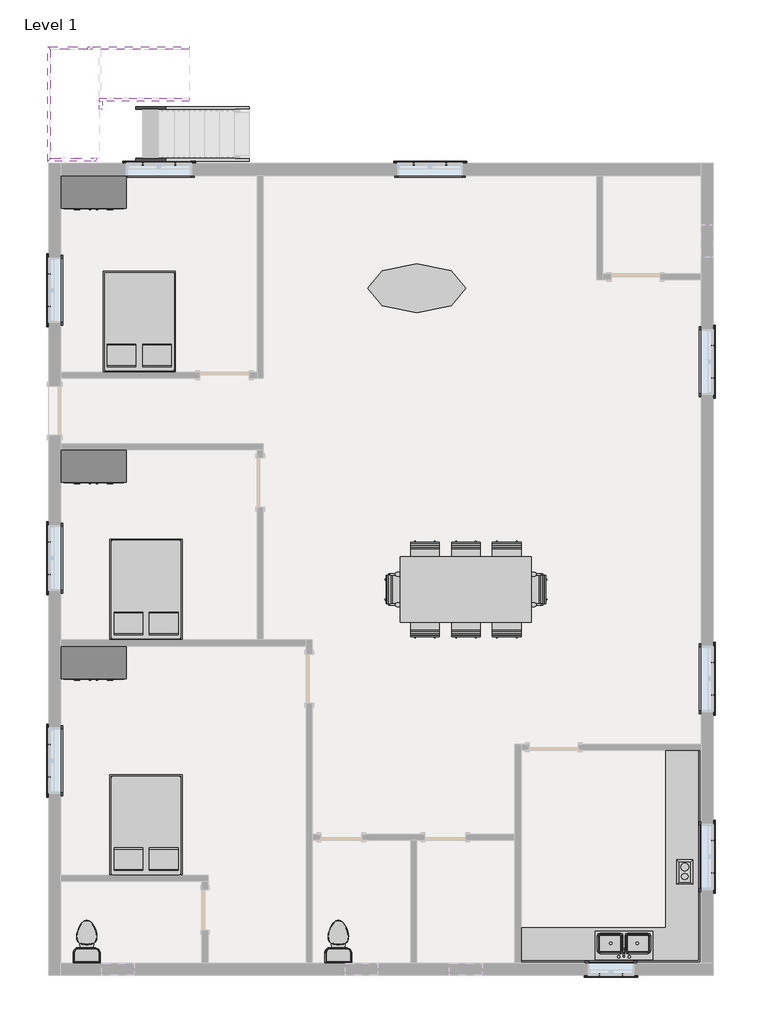
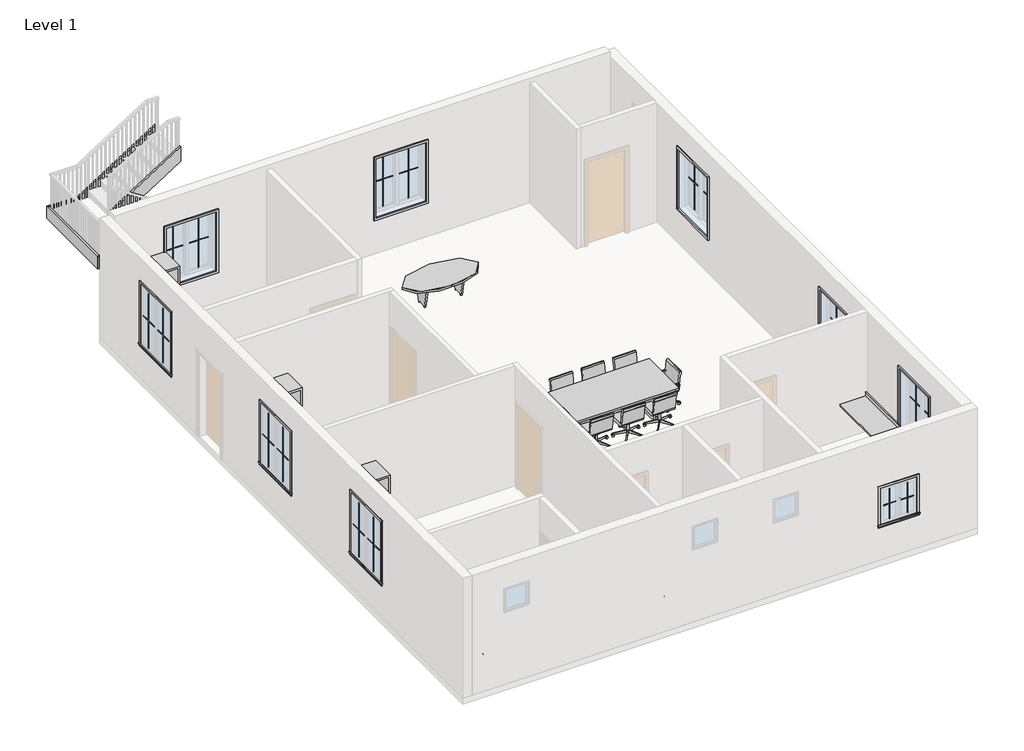
# One storey, part 3 of 3: 37 proxies, 17 furniture elements, 8 members, 3 flow terminals.
"""IFC4 building model written with IfcOpenShell, lengths in millimetres."""

from ifc_helpers import new_model, si_unit, frame, origin, place, context, project, spatial, polyline, outline, extrude, faceted_brep, transform, mapped, element, save
from components import proxy_fb8a77b2, muntin_pattern_2x2_muntin_pattern_2x2_6dad3731, muntin_pattern_2x2_muntin_pattern_2x2_a30a3345, muntin_pattern_2x2_muntin_pattern_2x2_b3fe6957, muntin_pattern_2x2_muntin_pattern_2x2_3e0ecaf2, trim_window_exterior_flat_with_sill_92b9b949, trim_window_exterior_flat_with_sill_41619996, trim_window_interior_flat_picture_frame_3bb882cf, trim_window_interior_flat_picture_frame_51c85655, flow_terminal_a53be723, toilet_domestic_3d_toilet_domestic_3d_ba6479b0, toilet_domestic_3d_toilet_domestic_3d_30431060, furniture_b58f7881, chair_task_chair_task_b7f3823b, chair_task_arms_chair_task_arms_fa5a08ef, furniture_9ea68cb4, furniture_6f689152, furniture_c045eb45, furniture_82e269c4

model = new_model("IFC4")

# Units and contexts
model_context = context("Model", 3, world=origin())
ifc_project = project(units=[si_unit("LENGTHUNIT", "METRE", prefix="MILLI")], contexts=[model_context])

# Site, building, storey
site = spatial("IfcSite", under=ifc_project)
building = spatial("IfcBuilding", under=site)
storey = spatial("IfcBuildingStorey", under=building, Name="Level 1", Elevation=0.0)

# Proxies
placement = place(None, origin())
proxy_shape = proxy_fb8a77b2(model_context)
element("IfcBuildingElementProxy", 1, Name="Cook Top-2 Unit : 12\" x 18\"", ObjectType="Cook Top-2 Unit : 12\" x 18\"", at=placement, inside=storey, context=model_context, shape_type="MappedRepresentation", body=[
    mapped(proxy_shape, transform((21379.2713581, 7569.2416109, 0.0), x_axis=(1.0, 0.0, 0.0), y_axis=(0.0, 1.0, 0.0), z_axis=(0.0, 0.0, 1.0))),
])
muntin_pattern_2x2_muntin_pattern_2x2_shape = muntin_pattern_2x2_muntin_pattern_2x2_6dad3731(model_context)
element("IfcBuildingElementProxy", 2, Name="Muntin Pattern_2x2 : Muntin Pattern_2x2", ObjectType="Muntin Pattern_2x2 : Muntin Pattern_2x2", at=placement, inside=storey, context=model_context, shape_type="MappedRepresentation", body=[
    mapped(muntin_pattern_2x2_muntin_pattern_2x2_shape, transform((9615.8963581, 18129.3539065, 984.25), x_axis=(0.0, 1.0, 0.0), y_axis=(-1.0, 0.0, 0.0), z_axis=(0.0, 0.0, 1.0))),
])
element("IfcBuildingElementProxy", 3, Name="Muntin Pattern_2x2 : Muntin Pattern_2x2", ObjectType="Muntin Pattern_2x2 : Muntin Pattern_2x2", at=placement, inside=storey, context=model_context, shape_type="MappedRepresentation", body=[
    mapped(muntin_pattern_2x2_muntin_pattern_2x2_shape, transform((11360.5588581, 20785.2414065, 984.25), x_axis=(1.0, 0.0, 0.0), y_axis=(0.0, 1.0, 0.0), z_axis=(0.0, 0.0, 1.0))),
])
element("IfcBuildingElementProxy", 4, Name="Muntin Pattern_2x2 : Muntin Pattern_2x2", ObjectType="Muntin Pattern_2x2 : Muntin Pattern_2x2", at=placement, inside=storey, context=model_context, shape_type="MappedRepresentation", body=[
    mapped(muntin_pattern_2x2_muntin_pattern_2x2_shape, transform((9615.8963581, 13138.2539065, 984.25), x_axis=(0.0, 1.0, 0.0), y_axis=(-1.0, 0.0, 0.0), z_axis=(0.0, 0.0, 1.0))),
])
element("IfcBuildingElementProxy", 5, Name="Muntin Pattern_2x2 : Muntin Pattern_2x2", ObjectType="Muntin Pattern_2x2 : Muntin Pattern_2x2", at=placement, inside=storey, context=model_context, shape_type="MappedRepresentation", body=[
    mapped(muntin_pattern_2x2_muntin_pattern_2x2_shape, transform((9615.8963581, 9366.3539065, 984.25), x_axis=(0.0, 1.0, 0.0), y_axis=(-1.0, 0.0, 0.0), z_axis=(0.0, 0.0, 1.0))),
])
element("IfcBuildingElementProxy", 6, Name="Muntin Pattern_2x2 : Muntin Pattern_2x2", ObjectType="Muntin Pattern_2x2 : Muntin Pattern_2x2", at=placement, inside=storey, context=model_context, shape_type="MappedRepresentation", body=[
    mapped(muntin_pattern_2x2_muntin_pattern_2x2_shape, transform((21979.3463581, 11496.7789065, 984.25), x_axis=(0.0, -1.0, 0.0), y_axis=(1.0, 0.0, 0.0), z_axis=(0.0, 0.0, 1.0))),
])
element("IfcBuildingElementProxy", 7, Name="Muntin Pattern_2x2 : Muntin Pattern_2x2", ObjectType="Muntin Pattern_2x2 : Muntin Pattern_2x2", at=placement, inside=storey, context=model_context, shape_type="MappedRepresentation", body=[
    mapped(muntin_pattern_2x2_muntin_pattern_2x2_shape, transform((21979.3463581, 17402.2789065, 984.25), x_axis=(0.0, -1.0, 0.0), y_axis=(1.0, 0.0, 0.0), z_axis=(0.0, 0.0, 1.0))),
])
element("IfcBuildingElementProxy", 8, Name="Muntin Pattern_2x2 : Muntin Pattern_2x2", ObjectType="Muntin Pattern_2x2 : Muntin Pattern_2x2", at=placement, inside=storey, context=model_context, shape_type="MappedRepresentation", body=[
    mapped(muntin_pattern_2x2_muntin_pattern_2x2_shape, transform((16408.8088581, 20785.2414065, 984.25), x_axis=(1.0, 0.0, 0.0), y_axis=(0.0, 1.0, 0.0), z_axis=(0.0, 0.0, 1.0))),
])
element("IfcBuildingElementProxy", 9, Name="Muntin Pattern_2x2 : Muntin Pattern_2x2", ObjectType="Muntin Pattern_2x2 : Muntin Pattern_2x2", at=placement, inside=storey, context=model_context, shape_type="MappedRepresentation", body=[
    mapped(muntin_pattern_2x2_muntin_pattern_2x2_shape, transform((21979.3463581, 8182.0789065, 984.25), x_axis=(0.0, -1.0, 0.0), y_axis=(1.0, 0.0, 0.0), z_axis=(0.0, 0.0, 1.0))),
])
muntin_pattern_2x2_muntin_pattern_2x2_2_shape = muntin_pattern_2x2_muntin_pattern_2x2_a30a3345(model_context)
element("IfcBuildingElementProxy", 10, Name="Muntin Pattern_2x2 : Muntin Pattern_2x2", ObjectType="Muntin Pattern_2x2 : Muntin Pattern_2x2", at=placement, inside=storey, context=model_context, shape_type="MappedRepresentation", body=[
    mapped(muntin_pattern_2x2_muntin_pattern_2x2_2_shape, transform((9615.8963581, 18735.7789065, 984.25), x_axis=(0.0, -1.0, 0.0), y_axis=(1.0, 0.0, 0.0), z_axis=(0.0, 0.0, 1.0))),
])
element("IfcBuildingElementProxy", 11, Name="Muntin Pattern_2x2 : Muntin Pattern_2x2", ObjectType="Muntin Pattern_2x2 : Muntin Pattern_2x2", at=placement, inside=storey, context=model_context, shape_type="MappedRepresentation", body=[
    mapped(muntin_pattern_2x2_muntin_pattern_2x2_2_shape, transform((11966.9838581, 20785.2414065, 984.25), x_axis=(-1.0, 0.0, 0.0), y_axis=(0.0, -1.0, 0.0), z_axis=(0.0, 0.0, 1.0))),
])
element("IfcBuildingElementProxy", 12, Name="Muntin Pattern_2x2 : Muntin Pattern_2x2", ObjectType="Muntin Pattern_2x2 : Muntin Pattern_2x2", at=placement, inside=storey, context=model_context, shape_type="MappedRepresentation", body=[
    mapped(muntin_pattern_2x2_muntin_pattern_2x2_2_shape, transform((9615.8963581, 13744.6789065, 984.25), x_axis=(0.0, -1.0, 0.0), y_axis=(1.0, 0.0, 0.0), z_axis=(0.0, 0.0, 1.0))),
])
element("IfcBuildingElementProxy", 13, Name="Muntin Pattern_2x2 : Muntin Pattern_2x2", ObjectType="Muntin Pattern_2x2 : Muntin Pattern_2x2", at=placement, inside=storey, context=model_context, shape_type="MappedRepresentation", body=[
    mapped(muntin_pattern_2x2_muntin_pattern_2x2_2_shape, transform((9615.8963581, 9972.7789065, 984.25), x_axis=(0.0, -1.0, 0.0), y_axis=(1.0, 0.0, 0.0), z_axis=(0.0, 0.0, 1.0))),
])
element("IfcBuildingElementProxy", 14, Name="Muntin Pattern_2x2 : Muntin Pattern_2x2", ObjectType="Muntin Pattern_2x2 : Muntin Pattern_2x2", at=placement, inside=storey, context=model_context, shape_type="MappedRepresentation", body=[
    mapped(muntin_pattern_2x2_muntin_pattern_2x2_2_shape, transform((21979.3463581, 10890.3539065, 984.25), x_axis=(0.0, 1.0, 0.0), y_axis=(-1.0, 0.0, 0.0), z_axis=(0.0, 0.0, 1.0))),
])
element("IfcBuildingElementProxy", 15, Name="Muntin Pattern_2x2 : Muntin Pattern_2x2", ObjectType="Muntin Pattern_2x2 : Muntin Pattern_2x2", at=placement, inside=storey, context=model_context, shape_type="MappedRepresentation", body=[
    mapped(muntin_pattern_2x2_muntin_pattern_2x2_2_shape, transform((21979.3463581, 16795.8539065, 984.25), x_axis=(0.0, 1.0, 0.0), y_axis=(-1.0, 0.0, 0.0), z_axis=(0.0, 0.0, 1.0))),
])
element("IfcBuildingElementProxy", 16, Name="Muntin Pattern_2x2 : Muntin Pattern_2x2", ObjectType="Muntin Pattern_2x2 : Muntin Pattern_2x2", at=placement, inside=storey, context=model_context, shape_type="MappedRepresentation", body=[
    mapped(muntin_pattern_2x2_muntin_pattern_2x2_2_shape, transform((17015.2338581, 20785.2414065, 984.25), x_axis=(-1.0, 0.0, 0.0), y_axis=(0.0, -1.0, 0.0), z_axis=(0.0, 0.0, 1.0))),
])
element("IfcBuildingElementProxy", 17, Name="Muntin Pattern_2x2 : Muntin Pattern_2x2", ObjectType="Muntin Pattern_2x2 : Muntin Pattern_2x2", at=placement, inside=storey, context=model_context, shape_type="MappedRepresentation", body=[
    mapped(muntin_pattern_2x2_muntin_pattern_2x2_2_shape, transform((21979.3463581, 7575.6539065, 984.25), x_axis=(0.0, 1.0, 0.0), y_axis=(-1.0, 0.0, 0.0), z_axis=(0.0, 0.0, 1.0))),
])
muntin_pattern_2x2_muntin_pattern_2x2_3_shape = muntin_pattern_2x2_muntin_pattern_2x2_b3fe6957(model_context)
element("IfcBuildingElementProxy", 18, Name="Muntin Pattern_2x2 : Muntin Pattern_2x2", ObjectType="Muntin Pattern_2x2 : Muntin Pattern_2x2", at=placement, inside=storey, context=model_context, shape_type="MappedRepresentation", body=[
    mapped(muntin_pattern_2x2_muntin_pattern_2x2_3_shape, transform((20298.1838581, 5678.5914065, 984.25), x_axis=(-1.0, 0.0, 0.0), y_axis=(0.0, -1.0, 0.0), z_axis=(0.0, 0.0, 1.0))),
])
muntin_pattern_2x2_muntin_pattern_2x2_4_shape = muntin_pattern_2x2_muntin_pattern_2x2_3e0ecaf2(model_context)
element("IfcBuildingElementProxy", 19, Name="Muntin Pattern_2x2 : Muntin Pattern_2x2", ObjectType="Muntin Pattern_2x2 : Muntin Pattern_2x2", at=placement, inside=storey, context=model_context, shape_type="MappedRepresentation", body=[
    mapped(muntin_pattern_2x2_muntin_pattern_2x2_4_shape, transform((19869.5588581, 5678.5914065, 984.25), x_axis=(1.0, 0.0, 0.0), y_axis=(0.0, 1.0, 0.0), z_axis=(0.0, 0.0, 1.0))),
])
trim_window_exterior_flat_with_sill_shape = trim_window_exterior_flat_with_sill_92b9b949(model_context)
element("IfcBuildingElementProxy", 20, Name="Trim-Window-Exterior-Flat : with Sill", ObjectType="Trim-Window-Exterior-Flat : with Sill", at=placement, inside=storey, context=model_context, shape_type="MappedRepresentation", body=[
    mapped(trim_window_exterior_flat_with_sill_shape, transform((9606.3713581, 18432.5664065, 2438.4), x_axis=(0.0, -1.0, 0.0), y_axis=(0.0, 0.0, 1.0), z_axis=(-1.0, 0.0, 0.0))),
])
element("IfcBuildingElementProxy", 21, Name="Trim-Window-Exterior-Flat : with Sill", ObjectType="Trim-Window-Exterior-Flat : with Sill", at=placement, inside=storey, context=model_context, shape_type="MappedRepresentation", body=[
    mapped(trim_window_exterior_flat_with_sill_shape, transform((11663.7713581, 20794.7664065, 2438.4), x_axis=(-1.0, 0.0, 0.0), y_axis=(0.0, 0.0, 1.0), z_axis=(0.0, 1.0, 0.0))),
])
element("IfcBuildingElementProxy", 22, Name="Trim-Window-Exterior-Flat : with Sill", ObjectType="Trim-Window-Exterior-Flat : with Sill", at=placement, inside=storey, context=model_context, shape_type="MappedRepresentation", body=[
    mapped(trim_window_exterior_flat_with_sill_shape, transform((9606.3713581, 13441.4664065, 2438.4), x_axis=(0.0, -1.0, 0.0), y_axis=(0.0, 0.0, 1.0), z_axis=(-1.0, 0.0, 0.0))),
])
element("IfcBuildingElementProxy", 23, Name="Trim-Window-Exterior-Flat : with Sill", ObjectType="Trim-Window-Exterior-Flat : with Sill", at=placement, inside=storey, context=model_context, shape_type="MappedRepresentation", body=[
    mapped(trim_window_exterior_flat_with_sill_shape, transform((9606.3713581, 9669.5664065, 2438.4), x_axis=(0.0, -1.0, 0.0), y_axis=(0.0, 0.0, 1.0), z_axis=(-1.0, 0.0, 0.0))),
])
element("IfcBuildingElementProxy", 24, Name="Trim-Window-Exterior-Flat : with Sill", ObjectType="Trim-Window-Exterior-Flat : with Sill", at=placement, inside=storey, context=model_context, shape_type="MappedRepresentation", body=[
    mapped(trim_window_exterior_flat_with_sill_shape, transform((21988.8713581, 11193.5664065, 2438.4), x_axis=(0.0, 1.0, 0.0), y_axis=(0.0, 0.0, 1.0), z_axis=(1.0, 0.0, 0.0))),
])
element("IfcBuildingElementProxy", 25, Name="Trim-Window-Exterior-Flat : with Sill", ObjectType="Trim-Window-Exterior-Flat : with Sill", at=placement, inside=storey, context=model_context, shape_type="MappedRepresentation", body=[
    mapped(trim_window_exterior_flat_with_sill_shape, transform((21988.8713581, 17099.0664065, 2438.4), x_axis=(0.0, 1.0, 0.0), y_axis=(0.0, 0.0, 1.0), z_axis=(1.0, 0.0, 0.0))),
])
element("IfcBuildingElementProxy", 26, Name="Trim-Window-Exterior-Flat : with Sill", ObjectType="Trim-Window-Exterior-Flat : with Sill", at=placement, inside=storey, context=model_context, shape_type="MappedRepresentation", body=[
    mapped(trim_window_exterior_flat_with_sill_shape, transform((16712.0213581, 20794.7664065, 2438.4), x_axis=(-1.0, 0.0, 0.0), y_axis=(0.0, 0.0, 1.0), z_axis=(0.0, 1.0, 0.0))),
])
element("IfcBuildingElementProxy", 27, Name="Trim-Window-Exterior-Flat : with Sill", ObjectType="Trim-Window-Exterior-Flat : with Sill", at=placement, inside=storey, context=model_context, shape_type="MappedRepresentation", body=[
    mapped(trim_window_exterior_flat_with_sill_shape, transform((21988.8713581, 7878.8664065, 2438.4), x_axis=(0.0, 1.0, 0.0), y_axis=(0.0, 0.0, 1.0), z_axis=(1.0, 0.0, 0.0))),
])
trim_window_exterior_flat_with_sill_2_shape = trim_window_exterior_flat_with_sill_41619996(model_context)
element("IfcBuildingElementProxy", 28, Name="Trim-Window-Exterior-Flat : with Sill", ObjectType="Trim-Window-Exterior-Flat : with Sill", at=placement, inside=storey, context=model_context, shape_type="MappedRepresentation", body=[
    mapped(trim_window_exterior_flat_with_sill_2_shape, transform((20083.8713581, 5669.0664065, 1828.8), x_axis=(1.0, 0.0, 0.0), y_axis=(0.0, 0.0, 1.0), z_axis=(0.0, -1.0, 0.0))),
])
trim_window_interior_flat_picture_frame_shape = trim_window_interior_flat_picture_frame_3bb882cf(model_context)
element("IfcBuildingElementProxy", 29, Name="Trim-Window-Interior-Flat : Picture Frame", ObjectType="Trim-Window-Interior-Flat : Picture Frame", at=placement, inside=storey, context=model_context, shape_type="MappedRepresentation", body=[
    mapped(trim_window_interior_flat_picture_frame_shape, transform((9834.9713581, 18432.5664065, 2438.4), x_axis=(0.0, 1.0, 0.0), y_axis=(0.0, 0.0, 1.0), z_axis=(1.0, 0.0, 0.0))),
])
element("IfcBuildingElementProxy", 30, Name="Trim-Window-Interior-Flat : Picture Frame", ObjectType="Trim-Window-Interior-Flat : Picture Frame", at=placement, inside=storey, context=model_context, shape_type="MappedRepresentation", body=[
    mapped(trim_window_interior_flat_picture_frame_shape, transform((11663.7713581, 20566.1664065, 2438.4), x_axis=(1.0, 0.0, 0.0), y_axis=(0.0, 0.0, 1.0), z_axis=(0.0, -1.0, 0.0))),
])
element("IfcBuildingElementProxy", 31, Name="Trim-Window-Interior-Flat : Picture Frame", ObjectType="Trim-Window-Interior-Flat : Picture Frame", at=placement, inside=storey, context=model_context, shape_type="MappedRepresentation", body=[
    mapped(trim_window_interior_flat_picture_frame_shape, transform((9834.9713581, 13441.4664065, 2438.4), x_axis=(0.0, 1.0, 0.0), y_axis=(0.0, 0.0, 1.0), z_axis=(1.0, 0.0, 0.0))),
])
element("IfcBuildingElementProxy", 32, Name="Trim-Window-Interior-Flat : Picture Frame", ObjectType="Trim-Window-Interior-Flat : Picture Frame", at=placement, inside=storey, context=model_context, shape_type="MappedRepresentation", body=[
    mapped(trim_window_interior_flat_picture_frame_shape, transform((9834.9713581, 9669.5664065, 2438.4), x_axis=(0.0, 1.0, 0.0), y_axis=(0.0, 0.0, 1.0), z_axis=(1.0, 0.0, 0.0))),
])
element("IfcBuildingElementProxy", 33, Name="Trim-Window-Interior-Flat : Picture Frame", ObjectType="Trim-Window-Interior-Flat : Picture Frame", at=placement, inside=storey, context=model_context, shape_type="MappedRepresentation", body=[
    mapped(trim_window_interior_flat_picture_frame_shape, transform((21760.2713581, 11193.5664065, 2438.4), x_axis=(0.0, -1.0, 0.0), y_axis=(0.0, 0.0, 1.0), z_axis=(-1.0, 0.0, 0.0))),
])
element("IfcBuildingElementProxy", 34, Name="Trim-Window-Interior-Flat : Picture Frame", ObjectType="Trim-Window-Interior-Flat : Picture Frame", at=placement, inside=storey, context=model_context, shape_type="MappedRepresentation", body=[
    mapped(trim_window_interior_flat_picture_frame_shape, transform((21760.2713581, 17099.0664065, 2438.4), x_axis=(0.0, -1.0, 0.0), y_axis=(0.0, 0.0, 1.0), z_axis=(-1.0, 0.0, 0.0))),
])
element("IfcBuildingElementProxy", 35, Name="Trim-Window-Interior-Flat : Picture Frame", ObjectType="Trim-Window-Interior-Flat : Picture Frame", at=placement, inside=storey, context=model_context, shape_type="MappedRepresentation", body=[
    mapped(trim_window_interior_flat_picture_frame_shape, transform((16712.0213581, 20566.1664065, 2438.4), x_axis=(1.0, 0.0, 0.0), y_axis=(0.0, 0.0, 1.0), z_axis=(0.0, -1.0, 0.0))),
])
element("IfcBuildingElementProxy", 36, Name="Trim-Window-Interior-Flat : Picture Frame", ObjectType="Trim-Window-Interior-Flat : Picture Frame", at=placement, inside=storey, context=model_context, shape_type="MappedRepresentation", body=[
    mapped(trim_window_interior_flat_picture_frame_shape, transform((21760.2713581, 7878.8664065, 2438.4), x_axis=(0.0, -1.0, 0.0), y_axis=(0.0, 0.0, 1.0), z_axis=(-1.0, 0.0, 0.0))),
])
trim_window_interior_flat_picture_frame_2_shape = trim_window_interior_flat_picture_frame_51c85655(model_context)
element("IfcBuildingElementProxy", 37, Name="Trim-Window-Interior-Flat : Picture Frame", ObjectType="Trim-Window-Interior-Flat : Picture Frame", at=placement, inside=storey, context=model_context, shape_type="MappedRepresentation", body=[
    mapped(trim_window_interior_flat_picture_frame_2_shape, transform((20083.8713581, 5897.6664065, 1828.8), x_axis=(-1.0, 0.0, 0.0), y_axis=(0.0, 0.0, 1.0), z_axis=(0.0, 1.0, 0.0))),
])

# Flow terminals
flow_terminal_shape = flow_terminal_a53be723(model_context)
element("IfcFlowTerminal", 38, ObjectType="Sink Kitchen-Double : 42\" x 21\"", at=placement, inside=storey, context=model_context, shape_type="MappedRepresentation", body=[
    mapped(flow_terminal_shape, transform((20340.8605987, 6230.2118076, 0.0), x_axis=(-1.0, 0.0, 0.0), y_axis=(0.0, -1.0, 0.0), z_axis=(0.0, 0.0, 1.0))),
])
toilet_domestic_3d_toilet_domestic_3d_shape = toilet_domestic_3d_toilet_domestic_3d_ba6479b0(model_context)
toilet_domestic_3d_toilet_domestic_3d_2_shape = toilet_domestic_3d_toilet_domestic_3d_30431060(model_context)
element("IfcFlowTerminal", 39, ObjectType="Toilet-Domestic-3D : Toilet-Domestic-3D", at=placement, inside=storey, context=model_context, shape_type="MappedRepresentation", body=[
    mapped(toilet_domestic_3d_toilet_domestic_3d_shape, transform((15003.8713581, 6392.3624338, 0.0), x_axis=(-1.0, 0.0, 0.0), y_axis=(0.0, -1.0, 0.0), z_axis=(0.0, 0.0, 1.0))),
    mapped(toilet_domestic_3d_toilet_domestic_3d_2_shape, transform((15003.8713581, 6392.3624338, 0.0), x_axis=(-1.0, 0.0, 0.0), y_axis=(0.0, -1.0, 0.0), z_axis=(0.0, 0.0, 1.0))),
])
element("IfcFlowTerminal", 40, ObjectType="Toilet-Domestic-3D : Toilet-Domestic-3D", at=placement, inside=storey, context=model_context, shape_type="MappedRepresentation", body=[
    mapped(toilet_domestic_3d_toilet_domestic_3d_shape, transform((10317.5713581, 6392.3624338, 0.0), x_axis=(-1.0, 0.0, 0.0), y_axis=(0.0, -1.0, 0.0), z_axis=(0.0, 0.0, 1.0))),
    mapped(toilet_domestic_3d_toilet_domestic_3d_2_shape, transform((10317.5713581, 6392.3624338, 0.0), x_axis=(-1.0, 0.0, 0.0), y_axis=(0.0, -1.0, 0.0), z_axis=(0.0, 0.0, 1.0))),
])

# Furniture
furniture_shape = furniture_b58f7881(model_context)
element("IfcFurniture", 41, ObjectType="Bed-Box : Double 53\" x 74\"", at=placement, inside=storey, context=model_context, shape_type="MappedRepresentation", body=[
    mapped(furniture_shape, transform((11636.4733436, 17613.9368983, 0.0), x_axis=(-1.0, 0.0, 0.0), y_axis=(0.0, -1.0, 0.0), z_axis=(0.0, 0.0, 1.0))),
])
element("IfcFurniture", 42, ObjectType="Bed-Box : Double 53\" x 74\"", at=placement, inside=storey, context=model_context, shape_type="MappedRepresentation", body=[
    mapped(furniture_shape, transform((11761.6238171, 12622.8368983, 0.0), x_axis=(-1.0, 0.0, 0.0), y_axis=(0.0, -1.0, 0.0), z_axis=(0.0, 0.0, 1.0))),
])
element("IfcFurniture", 43, ObjectType="Bed-Box : Double 53\" x 74\"", at=placement, inside=storey, context=model_context, shape_type="MappedRepresentation", body=[
    mapped(furniture_shape, transform((11761.6238171, 8228.6368983, 0.0), x_axis=(-1.0, 0.0, 0.0), y_axis=(0.0, -1.0, 0.0), z_axis=(0.0, 0.0, 1.0))),
])
chair_task_chair_task_shape = chair_task_chair_task_b7f3823b(model_context)
element("IfcFurniture", 44, ObjectType="Chair-Task : Chair-Task", at=placement, inside=storey, context=model_context, shape_type="MappedRepresentation", body=[
    mapped(chair_task_chair_task_shape, transform((17519.7621778, 13485.8123081, 0.0), x_axis=(-1.0, 0.0, 0.0), y_axis=(0.0, -1.0, 0.0), z_axis=(0.0, 0.0, 1.0))),
])
element("IfcFurniture", 45, ObjectType="Chair-Task : Chair-Task", at=placement, inside=storey, context=model_context, shape_type="MappedRepresentation", body=[
    mapped(chair_task_chair_task_shape, transform((18281.7621778, 13485.8123081, 0.0), x_axis=(-1.0, 0.0, 0.0), y_axis=(0.0, -1.0, 0.0), z_axis=(0.0, 0.0, 1.0))),
])
element("IfcFurniture", 46, ObjectType="Chair-Task : Chair-Task", at=placement, inside=storey, context=model_context, shape_type="MappedRepresentation", body=[
    mapped(chair_task_chair_task_shape, transform((17237.7805384, 12228.7205048, 0.0), x_axis=(1.0, 0.0, 0.0), y_axis=(0.0, 1.0, 0.0), z_axis=(0.0, 0.0, 1.0))),
])
element("IfcFurniture", 47, ObjectType="Chair-Task : Chair-Task", at=placement, inside=storey, context=model_context, shape_type="MappedRepresentation", body=[
    mapped(chair_task_chair_task_shape, transform((17999.7805384, 12228.7205048, 0.0), x_axis=(1.0, 0.0, 0.0), y_axis=(0.0, 1.0, 0.0), z_axis=(0.0, 0.0, 1.0))),
])
element("IfcFurniture", 48, ObjectType="Chair-Task : Chair-Task", at=placement, inside=storey, context=model_context, shape_type="MappedRepresentation", body=[
    mapped(chair_task_chair_task_shape, transform((16757.7621778, 13485.8123081, 0.0), x_axis=(-1.0, 0.0, 0.0), y_axis=(0.0, -1.0, 0.0), z_axis=(0.0, 0.0, 1.0))),
])
element("IfcFurniture", 49, ObjectType="Chair-Task : Chair-Task", at=placement, inside=storey, context=model_context, shape_type="MappedRepresentation", body=[
    mapped(chair_task_chair_task_shape, transform((16475.7805384, 12228.7205048, 0.0), x_axis=(1.0, 0.0, 0.0), y_axis=(0.0, 1.0, 0.0), z_axis=(0.0, 0.0, 1.0))),
])
chair_task_arms_chair_task_arms_shape = chair_task_arms_chair_task_arms_fa5a08ef(model_context)
element("IfcFurniture", 50, ObjectType="Chair-Task Arms : Chair-Task Arms", at=placement, inside=storey, context=model_context, shape_type="MappedRepresentation", body=[
    mapped(chair_task_arms_chair_task_arms_shape, transform((16140.6254565, 12998.2572261, 0.0), x_axis=(0.0, -1.0, 0.0), y_axis=(1.0, 0.0, 0.0), z_axis=(0.0, 0.0, 1.0))),
])
element("IfcFurniture", 51, ObjectType="Chair-Task Arms : Chair-Task Arms", at=placement, inside=storey, context=model_context, shape_type="MappedRepresentation", body=[
    mapped(chair_task_arms_chair_task_arms_shape, transform((18616.9172597, 12716.2755868, 0.0), x_axis=(0.0, 1.0, 0.0), y_axis=(-1.0, 0.0, 0.0), z_axis=(0.0, 0.0, 1.0))),
])
furniture_2_shape = furniture_9ea68cb4(model_context)
element("IfcFurniture", 52, ObjectType="Counter Top-L Shaped w Sink : 24\" Depth", at=placement, inside=storey, context=model_context, shape_type="MappedRepresentation", body=[
    mapped(furniture_2_shape, transform((20534.409063, 5923.0664065, 0.0), x_axis=(-1.0, 0.0, 0.0), y_axis=(0.0, -1.0, 0.0), z_axis=(0.0, 0.0, 1.0))),
])
furniture_3_shape = furniture_6f689152(model_context)
element("IfcFurniture", 53, ObjectType="Table-Conference2 w Chairs : 48\" x 144\"", at=placement, inside=storey, context=model_context, shape_type="MappedRepresentation", body=[
    mapped(furniture_3_shape, transform((17378.7713581, 12857.2664065, 0.0), x_axis=(1.0, 0.0, 0.0), y_axis=(0.0, 1.0, 0.0), z_axis=(0.0, 0.0, 1.0))),
])
furniture_4_shape = furniture_c045eb45(model_context)
element("IfcFurniture", 54, ObjectType="Table-Ellipse : 72\" x 36\"", at=placement, inside=storey, context=model_context, shape_type="MappedRepresentation", body=[
    mapped(furniture_4_shape, transform((16464.3713581, 18470.6664065, 0.0), x_axis=(1.0, 0.0, 0.0), y_axis=(0.0, 1.0, 0.0), z_axis=(0.0, 0.0, 1.0))),
])
furniture_5_shape = furniture_82e269c4(model_context)
element("IfcFurniture", 55, ObjectType="Wardrobe : 48\" x 72\" x 24\"", at=placement, inside=storey, context=model_context, shape_type="MappedRepresentation", body=[
    mapped(furniture_5_shape, transform((10713.7646179, 12082.105216, 0.0), x_axis=(1.0, 0.0, 0.0), y_axis=(0.0, 1.0, 0.0), z_axis=(0.0, 0.0, 1.0))),
])
element("IfcFurniture", 56, ObjectType="Wardrobe : 48\" x 72\" x 24\"", at=placement, inside=storey, context=model_context, shape_type="MappedRepresentation", body=[
    mapped(furniture_5_shape, transform((10713.7646179, 15739.705216, 0.0), x_axis=(1.0, 0.0, 0.0), y_axis=(0.0, 1.0, 0.0), z_axis=(0.0, 0.0, 1.0))),
])
element("IfcFurniture", 57, ObjectType="Wardrobe : 48\" x 72\" x 24\"", at=placement, inside=storey, context=model_context, shape_type="MappedRepresentation", body=[
    mapped(furniture_5_shape, transform((10713.7646179, 20845.105216, 0.0), x_axis=(1.0, 0.0, 0.0), y_axis=(0.0, 1.0, 0.0), z_axis=(0.0, 0.0, 1.0))),
])

# Members
element("IfcMember", 58, ObjectType="Stringer - 2\" Width", at=placement, inside=storey, context=model_context, shape_type="SweptSolid", body=[
    extrude(outline(polyline([(0.0, 13347.9752377), (215.0106437, 13347.9752377), (2032.0, 10492.7062492), (1727.2, 10403.9482797), (0.0, 13118.1197083), (0.0, 13347.9752377)])), frame((0.0, 20836.0384539, 0.0), z_axis=(0.0, 1.0, 0.0), x_axis=(0.0, 0.0, 1.0)), (0.0, 0.0, 1.0), 50.8),
])
element("IfcMember", 59, ObjectType="Stringer - 2\" Width", at=placement, inside=storey, context=model_context, shape_type="SweptSolid", body=[
    extrude(outline(polyline([(0.0, 13347.9752377), (215.0106437, 13347.9752377), (1960.683371, 10604.7752377), (1599.4010268, 10604.7752377), (0.0, 13118.1197083), (0.0, 13347.9752377)])), frame((0.0, 21801.2384539, 0.0), z_axis=(0.0, 1.0, 0.0), x_axis=(0.0, 0.0, 1.0)), (0.0, 0.0, 1.0), 50.8),
])
element("IfcMember", 60, ObjectType="Stringer - 2\" Width", at=placement, inside=storey, context=model_context, shape_type="SweptSolid", body=[
    extrude(outline(polyline([(2032.0, 10335.8442261), (1727.2, 10424.6021956), (2876.3282995, 12230.3752377), (3237.6106437, 12230.3752377), (2032.0, 10335.8442261)])), frame((0.0, 22920.6919009, 0.0), z_axis=(0.0, 1.0, 0.0), x_axis=(0.0, 0.0, 1.0)), (0.0, 0.0, 1.0), 50.8),
])
element("IfcMember", 61, ObjectType="Stringer - 2\" Width", at=placement, inside=storey, context=model_context, shape_type="SweptSolid", body=[
    extrude(outline(polyline([(2170.8106437, 10553.9752377), (1809.5282995, 10553.9752377), (2876.3282995, 12230.3752377), (3237.6106437, 12230.3752377), (2170.8106437, 10553.9752377)])), frame((0.0, 21955.4919009, 0.0), z_axis=(0.0, 1.0, 0.0), x_axis=(0.0, 0.0, 1.0)), (0.0, 0.0, 1.0), 50.8),
])
element("IfcMember", 62, ObjectType="Stringer - 2\" Width", at=placement, inside=storey, context=model_context, shape_type="Brep", body=[
    faceted_brep([(10335.8442261, 22920.6919009, 2032.0), (10335.8442261, 22971.4919009, 2032.0), (9588.7752377, 22971.4919009, 2032.0), (9639.5752377, 22920.6919009, 2032.0), (10424.6021956, 22920.6919009, 1727.2), (9639.5752377, 22920.6919009, 1727.2), (10424.6021956, 22971.4919009, 1727.2), (9588.7752377, 22971.4919009, 1727.2)], [[[0, 1, 2, 3]], [[4, 0, 3, 5]], [[6, 4, 5, 7]], [[1, 6, 7, 2]], [[1, 0, 4, 6]], [[2, 7, 5, 3]]]),
])
element("IfcMember", 63, ObjectType="Stringer - 2\" Width", at=placement, inside=storey, context=model_context, shape_type="SweptSolid", body=[
    extrude(outline(polyline([(9588.7752377, 22971.4919009), (9639.5752377, 22920.6919009), (9639.5752377, 20886.8384539), (9588.7752377, 20836.0384539), (9588.7752377, 22971.4919009)])), frame((0.0, 0.0, 1727.2), z_axis=(0.0, 0.0, 1.0), x_axis=(1.0, 0.0, 0.0)), (0.0, 0.0, 1.0), 304.8),
])
element("IfcMember", 64, ObjectType="Stringer - 2\" Width", at=placement, inside=storey, context=model_context, shape_type="Brep", body=[
    faceted_brep([(9639.5752377, 20886.8384539, 2032.0), (9588.7752377, 20836.0384539, 2032.0), (10492.7062492, 20836.0384539, 2032.0), (10492.7062492, 20886.8384539, 2032.0), (9639.5752377, 20886.8384539, 1727.2), (10403.9482797, 20886.8384539, 1727.2), (9588.7752377, 20836.0384539, 1727.2), (10403.9482797, 20836.0384539, 1727.2)], [[[0, 1, 2, 3]], [[4, 0, 3, 5]], [[6, 4, 5, 7]], [[1, 6, 7, 2]], [[1, 0, 4, 6]], [[2, 7, 5, 3]]]),
])
element("IfcMember", 65, ObjectType="Stringer - 2\" Width", at=placement, inside=storey, context=model_context, shape_type="SweptSolid", body=[
    extrude(outline(polyline([(10604.7752377, 21801.2384539), (10553.9752377, 21801.2384539), (10553.9752377, 21955.4919009), (10604.7752377, 21955.4919009), (10604.7752377, 21801.2384539)])), frame((0.0, 0.0, 1727.2), z_axis=(0.0, 0.0, 1.0), x_axis=(1.0, 0.0, 0.0)), (0.0, 0.0, 1.0), 304.8),
])

save(model, "model.ifc")

# Revit data of these elements
# Type "Cook Top-2 Unit : 12\" x 18\""
#   Assembly Code = "E1090400"
#   Counter Height = 3' - 0"
#   Depth = 1' - 6"
#   Width = 1' - 0"
#   Burner Material = Metal - Chrome
#   Cooktop Material = Metal - Steel, Polished
#   Default Elevation = 0
# Type "Muntin Pattern_2x2 : Muntin Pattern_2x2"
#   Width [instance default] = 4' - 0"
#   Thickness = 0' - 0 1/2"
#   Height [instance default] = 4' - 0"
#   Distance = 0' - 0 3/4"
#   Interior Material [instance default] = none
#   Exterior Material [instance default] = none
#   Default Elevation = 0
# Type "Trim-Window-Exterior-Flat : with Sill"
#   Trim Width = 0' - 2 1/4"
#   Trim Thickness_Picture Frame = 0' - 1 1/4"
#   Trim Thickness_with Sill = 0' - 0 3/4"
#   Sill Thickness = 0' - 1 1/4"
#   Opening Width [instance default] = 2' - 0"
#   Opening Height [instance default] = 3' - 0"
#   Default Elevation = 4' - 0"
#   Sill = yes
#   Picture Frame = no
#   Trim Material [instance default] = none
# Type "Trim-Window-Interior-Flat : Picture Frame"
#   Trim Thickness_Picture Frame = 0' - 1 1/4"
#   Trim Width = 0' - 2 1/4"
#   Trim Thickness_with Sill = 0' - 0 3/4"
#   Sill Thickness = 0' - 1 1/4"
#   Opening Width [instance default] = 2' - 0"
#   Opening Height [instance default] = 3' - 0"
#   Default Elevation = 4' - 0"
#   Sill = no
#   Picture Frame = yes
#   Trim Material [instance default] = none
# Type "Sink Kitchen-Double : 42\" x 21\""
#   Assembly Code = "D2010410"
#   Counter Height = 3' - 0"
#   Depth = 1' - 9"
#   Width = 3' - 6"
#   Faucet Material = Steel, Polished
#   Sink Material = Steel, Polished
#   Default Elevation = 0
# Type "Toilet-Domestic-3D : Toilet-Domestic-3D"
#   Assembly Code = "D2010110"
#   Toilet - Bowl/Basin Material = Porcelain, Linen
#   Toilet - Seat Material = Laminate, Linen, Matte
#   Default Elevation = 0
# Type "Bed-Box : Double 53\" x 74\""
#   Assembly Code = "E2020200"
#   Length = 6' - 2"
#   Width = 4' - 5"
#   Frame Material = Birch
#   Mattress Material = Linen, White
#   Default Elevation = 0
# Type "Chair-Task : Chair-Task"
#   Assembly Code = "E2020200"
#   Base Material = Plastic - Black
#   Caster Material = Plastic - Black
#   Seat/Back Material = Textile - Slate Blue
#   Default Elevation = 0
# Type "Chair-Task Arms : Chair-Task Arms"
#   Assembly Code = "E2020200"
#   Base Material = Plastic - Black
#   Caster Material = Plastic - Black
#   Seat/Back Material = Textile - Slate Blue
#   Default Elevation = 0
# Type "Counter Top-L Shaped w Sink : 24\" Depth"
#   Assembly Code = "C1030400"
#   Counter Thickness = 0' - 1 1/2"
#   Depth = 2' - 1"
#   Height = 3' - 0"
#   Length - Leg 1 [instance default] = 8' - 0"
#   Length - Leg 2 [instance default] = 6' - 0"
#   Sink Location [instance default] = 3' - 0"
#   Sink Location To Wall [instance default] = 0' - 6"
#   Sink Opening Depth [instance default] = 1' - 3"
#   Sink Opening Width [instance default] = 3' - 3"
#   Counter Top Material = none
#   Default Elevation = 0
# Type "Table-Conference2 w Chairs : 48\" x 144\""
#   Assembly Code = "E2020200"
#   Description = "Seating 12-14"
#   Height = 2' - 6"
#   Length = 8' - 0"
#   Width = 4' - 0"
#   Number Of Chairs One Side = 3
#   Number Of Chairs = 8
#   Material = Wood - Cherry
#   Default Elevation = 0
# Type "Table-Ellipse : 72\" x 36\""
#   Assembly Code = "E2020200"
#   Half Width = 1' - 6"
#   Half Length = 3' - 0"
#   Height = 2' - 0"
#   Length = 6' - 0"
#   Width = 3' - 0"
#   Base Material = Birch
#   Top Material = Laminate - Black
#   Default Elevation = 0
# Type "Wardrobe : 48\" x 72\" x 24\""
#   Assembly Code = "E2020200"
#   Depth = 2' - 0"
#   Height = 6' - 0"
#   Width = 4' - 0"
#   Material = Wood - Mahogany
#   Default Elevation = 0
# Element 1 (IfcBuildingElementProxy, "Cook Top-2 Unit : 12\" x 18\"")
#   Phase Created = New Construction
#   Materials on its faces: "Metal - Steel, Polished", "Metal - Chrome"
# Elements 2, 3, 4, 5, 6, 7, 8, 9, 10, 11, 12, 13, 14, 15, 16, 17 (IfcBuildingElementProxy, "Muntin Pattern_2x2 : Muntin Pattern_2x2")
#   Width = 1' - 6 5/8"
#   Height = 4' - 6 1/2"
#   Interior Material = Wood - Stained
#   Exterior Material = Clad - White
#   Phase Created = New Construction
#   Materials on its faces: "Clad - White", "Wood - Stained"
# Elements 18, 19 (IfcBuildingElementProxy, "Muntin Pattern_2x2 : Muntin Pattern_2x2")
#   Width = 0' - 11 5/8"
#   Height = 2' - 6 1/2"
#   Interior Material = Wood - Stained
#   Exterior Material = Clad - White
#   Phase Created = New Construction
#   Materials on its faces: "Clad - White", "Wood - Stained"
# Elements 20, 21, 22, 23, 24, 25, 26, 27 (IfcBuildingElementProxy, "Trim-Window-Exterior-Flat : with Sill")
#   Opening Width = 4' - 0"
#   Opening Height = 5' - 0"
#   Trim Material = Clad - White
#   Phase Created = New Construction
#   Materials on its faces: "Clad - White"
# Element 28 (IfcBuildingElementProxy, "Trim-Window-Exterior-Flat : with Sill")
#   Opening Width = 2' - 10"
#   Opening Height = 3' - 0"
#   Trim Material = Clad - White
#   Phase Created = New Construction
#   Materials on its faces: "Clad - White"
# Elements 29, 30, 31, 32, 33, 34, 35, 36 (IfcBuildingElementProxy, "Trim-Window-Interior-Flat : Picture Frame")
#   Opening Width = 4' - 0"
#   Opening Height = 5' - 0"
#   Trim Material = Wood - Stained
#   Phase Created = New Construction
#   Materials on its faces: "Wood - Stained"
# Element 37 (IfcBuildingElementProxy, "Trim-Window-Interior-Flat : Picture Frame")
#   Opening Width = 2' - 10"
#   Opening Height = 3' - 0"
#   Trim Material = Wood - Stained
#   Phase Created = New Construction
#   Materials on its faces: "Wood - Stained"
# Element 38 (IfcFlowTerminal, "Sink Kitchen-Double : 42\" x 21\"")
#   Mark = "2"
#   Phase Created = New Construction
#   Materials on its faces: "Steel, Polished"
# Element 39 (IfcFlowTerminal, "Toilet-Domestic-3D : Toilet-Domestic-3D")
#   Mark = "1"
#   Phase Created = New Construction
#   Materials on its faces: "Porcelain, Linen", "Laminate, Linen, Matte"
# Element 40 (IfcFlowTerminal, "Toilet-Domestic-3D : Toilet-Domestic-3D")
#   Mark = "3"
#   Phase Created = New Construction
#   Materials on its faces: "Porcelain, Linen", "Laminate, Linen, Matte"
# Elements 41, 42, 43 (IfcFurniture, "Bed-Box : Double 53\" x 74\"")
#   Phase Created = New Construction
#   Materials on its faces: "Birch", "Linen, White"
# Elements 44, 45, 46, 47, 48, 49 (IfcFurniture, "Chair-Task : Chair-Task")
#   Phase Created = New Construction
#   Materials on its faces: "Plastic - Black", "Textile - Slate Blue"
# Elements 50, 51 (IfcFurniture, "Chair-Task Arms : Chair-Task Arms")
#   Phase Created = New Construction
#   Materials on its faces: "Plastic - Black", "Textile - Slate Blue"
# Element 52 (IfcFurniture, "Counter Top-L Shaped w Sink : 24\" Depth")
#   Sink Opening Width = 3' - 3"
#   Sink Opening Depth = 1' - 3"
#   Sink Location To Wall = 0' - 6"
#   Sink Location = 3' - 0"
#   Length - Leg 2 = 12' - 11"
#   Length - Leg 1 = 10' - 11"
#   Phase Created = New Construction
#   Materials on its faces: "Counter Top"
# Element 53 (IfcFurniture, "Table-Conference2 w Chairs : 48\" x 144\"")
#   Phase Created = New Construction
#   Materials on its faces: "Wood - Cherry"
# Element 54 (IfcFurniture, "Table-Ellipse : 72\" x 36\"")
#   Phase Created = New Construction
#   Materials on its faces: "Birch", "Laminate - Black"
# Elements 55, 56, 57 (IfcFurniture, "Wardrobe : 48\" x 72\" x 24\"")
#   Phase Created = New Construction
#   Materials on its faces: "Wood - Mahogany"
# Elements 58, 59, 60, 61, 62, 63, 64, 65 (IfcMember, "Stringer - 2\" Width")
#   Phase Created = New Construction
# Materials
#   "Metal - Chrome": class "Metal", colour RGB 247 247 247, transparency 0
#   "Metal - Steel, Polished": colour RGB 57 57 57, transparency 0
#   "Steel, Polished": class "Metal", colour RGB 192 192 192, transparency 0, Description = "Polished steel", Cost = 0
#   "Porcelain, Linen": class "Ceramic", colour RGB 249 239 230, transparency 0, Description = "Porcelain, linen", Cost = 0
#   "Laminate, Linen, Matte": class "Plastic", colour RGB 249 239 230, transparency 0, Description = "Plastic Laminate - Linen, Matte", Cost = 0
#   "Birch": class "Wood", colour RGB 224 178 126, transparency 0, Description = "Betula Alleghaniensis", Cost = 0
#   "Linen, White": class "Textile", colour RGB 247 247 239, transparency 0, Description = "Linen, white", Cost = 0
#   "Plastic - Black": colour RGB 0 0 0, transparency 0.7
#   "Textile - Slate Blue": colour RGB 98 102 118, transparency 0
#   "Wood - Cherry": colour RGB 151 75 0, transparency 0
#   "Laminate - Black": colour RGB 0 0 0, transparency 0
#   "Wood - Mahogany": colour RGB 138 86 45, transparency 0
#   "Clad - White": class "Wood", colour RGB 242 242 238, transparency 0, Cost = 0
#   "Wood - Stained": class "Wood", colour RGB 224 178 126, transparency 0, Cost = 0
#   "Counter Top": class "Wood", colour RGB 226 177 128, transparency 0
